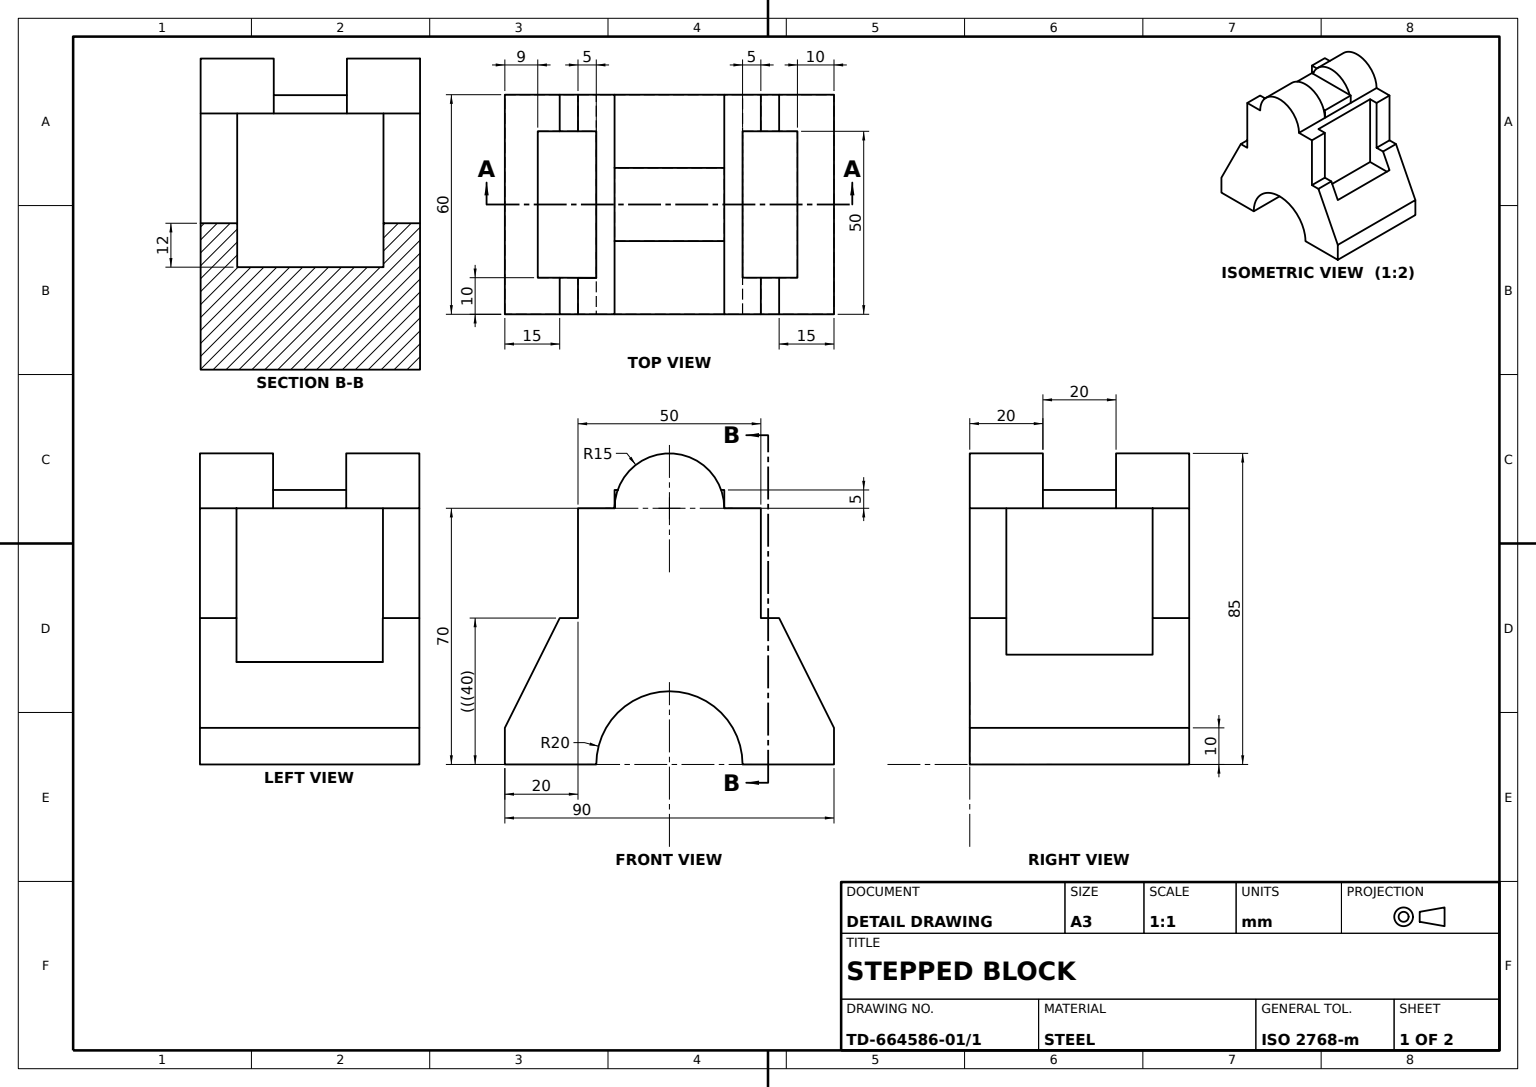
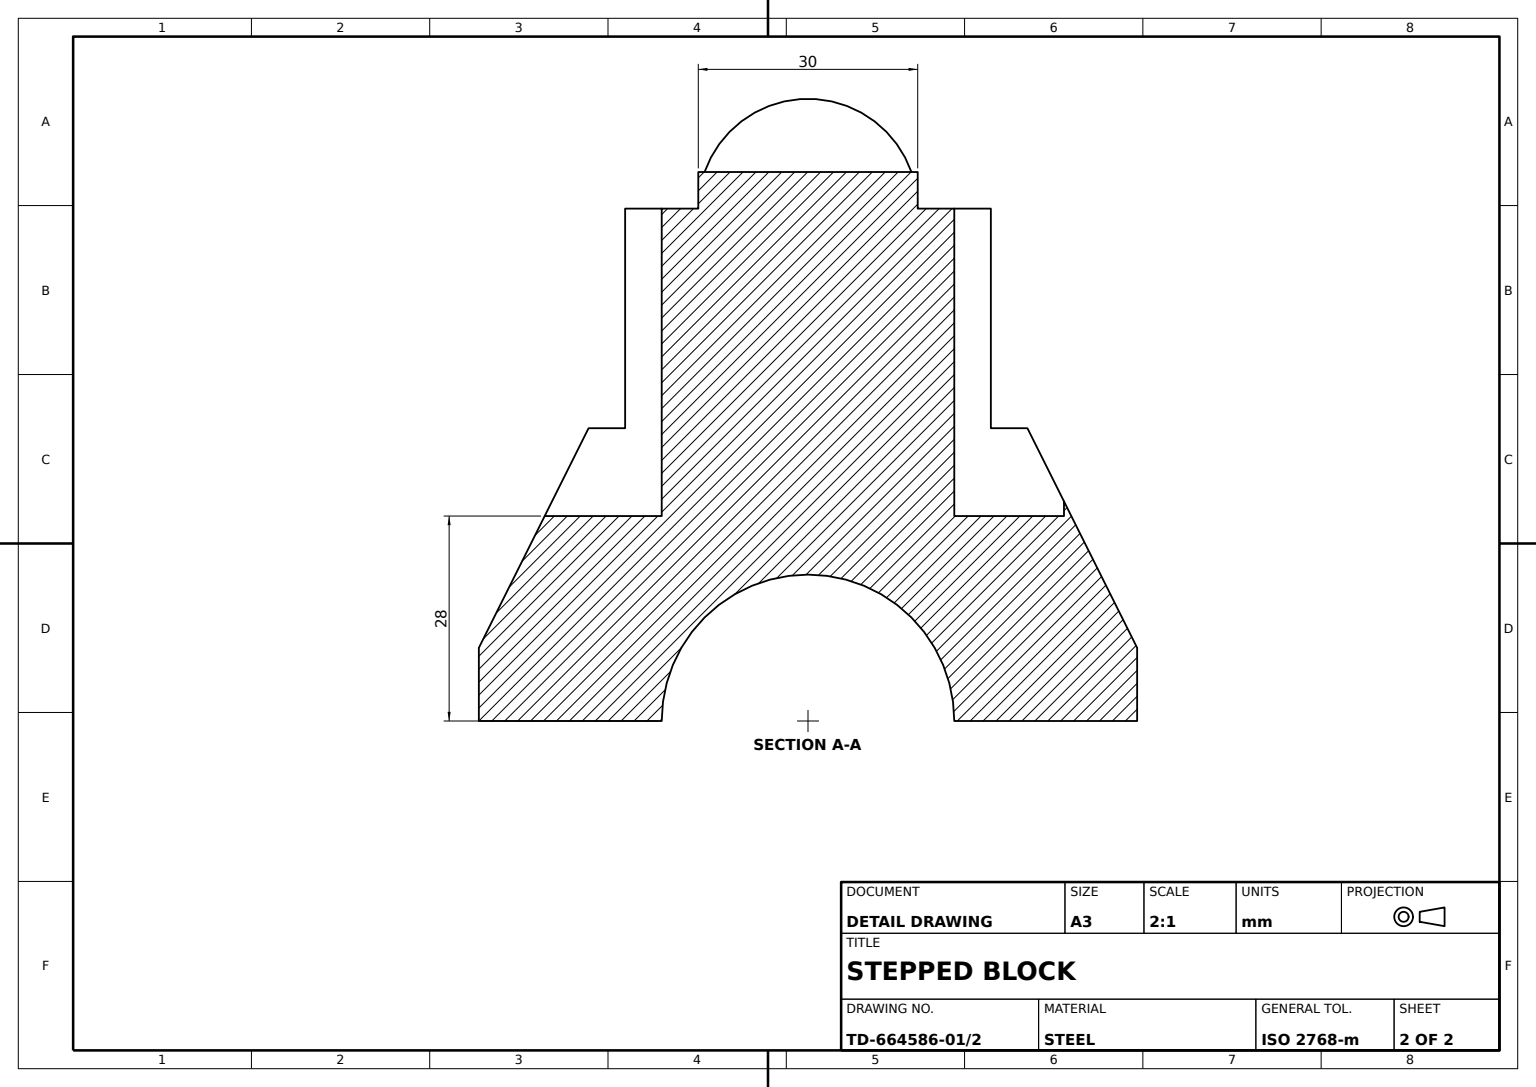
from build123d import *

# Parameters (mm, degrees)
ARCHED_BODY_60_DEPTH         = 60
POCKET_A_STEP_CUT_5_DEPTH    = 5
POCKET_A_CUT_12_DEPTH        = 12
POCKET_B_STEP_CUT_5_DEPTH    = 5
POCKET_B_SKETCH_W            = 15
POCKET_B_SKETCH_H            = 40
POCKET_B_CUT_12_DEPTH        = 12
TOP_HALF_ROUND_CUT_40_DEPTH  = 40
TOP_PAD_SKETCH_W             = 30
TOP_PAD_SKETCH_H             = 20
TOP_PAD_5_DEPTH              = 5
TOP_HALF_ROUND_BOSS_20_DEPTH = 20


with BuildPart() as part:
    # Arched Body Profile Sketch → Arched Body 60 (new body)
    with BuildSketch(Plane.XY):
        with BuildLine():
            Line((0, 0), (25, 0))
            ThreePointArc((25, 0), (45, 20), (65, 0))
            Line((65, 0), (90, 0))
            Line((90, 0), (90, 10))
            Line((90, 10), (75, 40))
            Line((75, 40), (70, 40))
            Line((70, 40), (70, 70))
            Line((70, 70), (60, 70))
            ThreePointArc((60, 70), (45, 85), (30, 70))
            Line((30, 70), (20, 70))
            Line((20, 70), (20, 40))
            Line((20, 40), (15, 40))
            Line((15, 40), (0, 10))
            Line((0, 10), (0, 0))
        make_face()
    extrude(amount=ARCHED_BODY_60_DEPTH)

    # Pocket A Step Sketch → Pocket A Step Cut 5 (cut)
    with BuildSketch(Plane.ZY.offset(-20)):
        Polygon((30, 70), (10, 70), (10, 40), (50.046888812, 40), (50.046888812, 70), align=None)
    extrude(amount=-POCKET_A_STEP_CUT_5_DEPTH, mode=Mode.SUBTRACT)

    # Pocket A Sketch → Pocket A Cut 12 (cut)
    with BuildSketch(Plane(origin=(0, 40, 0), x_dir=(1, 0, 0), z_dir=(0, 1, 0))):
        Polygon((20, -10), (15, -10), (5, -10), (5, -50), (15, -50), (25, -50.046888812), (25, -10), align=None)
    extrude(amount=-POCKET_A_CUT_12_DEPTH, mode=Mode.SUBTRACT)

    # Pocket B Step Sketch → Pocket B Step Cut 5 (cut)
    with BuildSketch(Plane(origin=(70, 0, 0), x_dir=(0, 0, -1), z_dir=(1, 0, 0))):
        Polygon((-30, 70), (-50, 70), (-50, 40), (-10, 40), (-10, 70), align=None)
    extrude(amount=-POCKET_B_STEP_CUT_5_DEPTH, mode=Mode.SUBTRACT)

    # Pocket B Sketch → Pocket B Cut 12 (cut)
    with BuildSketch(Plane(origin=(0, 40, 0), x_dir=(1, 0, 0), z_dir=(0, 1, 0))):
        with Locations((72.5, -30)):
            Rectangle(POCKET_B_SKETCH_W, POCKET_B_SKETCH_H)
    extrude(amount=-POCKET_B_CUT_12_DEPTH, mode=Mode.SUBTRACT)

    # Top Half-Round Cut Sketch → Top Half-Round Cut 40 (cut)
    with BuildSketch(Plane(origin=(0, 0, 0), x_dir=(-1, 0, 0), z_dir=(0, 0, -1))):
        with BuildLine():
            Line((-60, 70), (-30, 70))
            ThreePointArc((-30, 70), (-45, 85), (-60, 70))
        make_face()
    extrude(amount=-TOP_HALF_ROUND_CUT_40_DEPTH, mode=Mode.SUBTRACT)

    # Top Pad Sketch → Top Pad 5 (add)
    with BuildSketch(Plane(origin=(0, 70, 0), x_dir=(1, 0, 0), z_dir=(0, 1, 0))):
        with Locations((45, -30)):
            Rectangle(TOP_PAD_SKETCH_W, TOP_PAD_SKETCH_H)
    extrude(amount=TOP_PAD_5_DEPTH)

    # Top Half-Round Boss Sketch → Top Half-Round Boss 20 (add)
    with BuildSketch(Plane(origin=(0, 0, 0), x_dir=(-1, 0, 0), z_dir=(0, 0, -1))):
        with BuildLine():
            Line((-60, 70), (-30, 70))
            ThreePointArc((-30, 70), (-45, 85), (-60, 70))
        make_face()
    extrude(amount=-TOP_HALF_ROUND_BOSS_20_DEPTH)


solid = part.part
